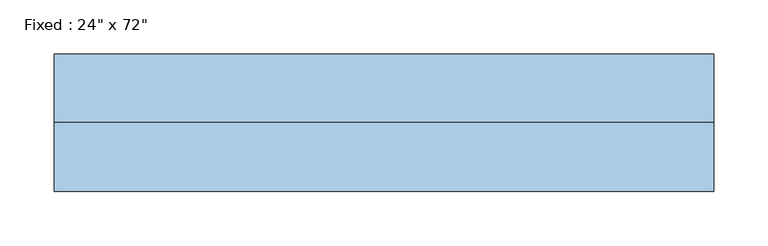
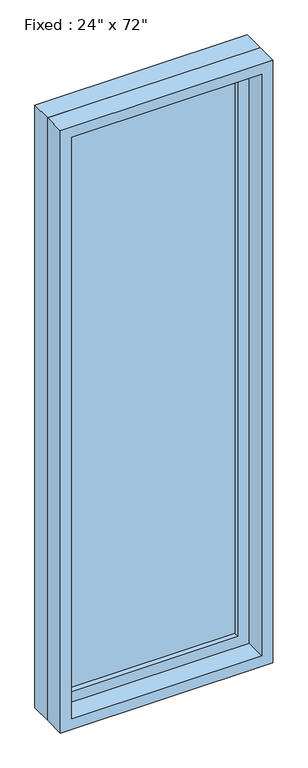
"""IFC4 building model written with IfcOpenShell, lengths in millimetres: window geometry."""

from ifc_helpers import new_model, si_unit, frame, origin, place, context, project, spatial, polyline, outline, extrude, source, transform, mapped, element, save


def window_0bf3737e(model_context):
    return source(origin(), model_context, "Body", "SweptSolid", [
        extrude(outline(polyline([(203.2, 15.875), (-279.4, 15.875), (-279.4, 28.575), (203.2, 28.575), (203.2, 15.875)])), frame((0.0, 0.0, 368.3), z_axis=(0.0, 0.0, 1.0), x_axis=(1.0, 0.0, 0.0)), (0.0, 0.0, 1.0), 1701.8),
        extrude(outline(polyline([(2114.55, -323.85), (323.85, -323.85), (323.85, 247.65), (2114.55, 247.65), (2114.55, -323.85)]), holes=[polyline([(2070.1, -279.4), (2070.1, 203.2), (368.3, 203.2), (368.3, -279.4), (2070.1, -279.4)])]), frame((0.0, 0.0, 0.0), z_axis=(0.0, 1.0, 0.0), x_axis=(0.0, 0.0, 1.0)), (0.0, 0.0, 1.0), 44.45),
        extrude(outline(polyline([(2133.6, -342.9), (304.8, -342.9), (304.8, 266.7), (2133.6, 266.7), (2133.6, -342.9)]), holes=[polyline([(2101.85, -311.15), (2101.85, 234.95), (336.55, 234.95), (336.55, -311.15), (2101.85, -311.15)])]), frame((0.0, -63.5, 0.0), z_axis=(0.0, 1.0, 0.0), x_axis=(0.0, 0.0, 1.0)), (0.0, 0.0, 1.0), 63.5),
        extrude(outline(polyline([(2133.6, 266.7), (2133.6, -342.9), (304.8, -342.9), (304.8, 266.7), (2133.6, 266.7)]), holes=[polyline([(2114.55, 247.65), (323.85, 247.65), (323.85, -323.85), (2114.55, -323.85), (2114.55, 247.65)])]), frame((0.0, 0.0, 0.0), z_axis=(0.0, 1.0, 0.0), x_axis=(0.0, 0.0, 1.0)), (0.0, 0.0, 1.0), 63.5),
    ])


if __name__ == "__main__":
    model = new_model("IFC4")
    model_context = context("Model", 3, world=origin())
    ifc_project = project(units=[si_unit("LENGTHUNIT", "METRE", prefix="MILLI")], contexts=[model_context])
    site = spatial("IfcSite", under=ifc_project)
    building = spatial("IfcBuilding", under=site)
    placement = place(None, origin())
    window_shape = window_0bf3737e(model_context)
    element("IfcWindow", 1, ObjectType="Fixed : 24\" x 72\"", at=placement, inside=building, context=model_context, shape_type="MappedRepresentation", body=[
        mapped(window_shape, transform((0.0, 0.0, 0.0), x_axis=(1.0, 0.0, 0.0), y_axis=(0.0, 1.0, 0.0), z_axis=(0.0, 0.0, 1.0))),
    ])
    save(model, "model.ifc")

# Revit data of these elements
# Type "Fixed : 24\" x 72\""
#   Type Mark = "7"
#   Construction Type Id = "GSP4R"
#   Assembly Code = "B2020100"
#   Analytic Construction = "1/8 in Pilkington single glazing"
#   Visual Light Transmittance = 0.9
#   Solar Heat Gain Coefficient = 0.78
#   Heat Transfer Coefficient (U) = 0.6496 BTU/(h·ft²·°F)
#   Height = 6' - 0"
#   Default Sill Height = 1' - 0"
#   Width = 2' - 0"
#   Window Inset = 0' - 0 3/4"
#   Define Thermal Properties by = 1
#   Define Thermal Properties by = 1
#   Glass Pane Material = Glass
#   Sash Material = Sash
#   Wall Closure = (empty or 0)
# Element 1 (IfcWindow, "Fixed : 24\" x 72\"")
#   Materials on its faces: "Sash", "Glass"
# Materials
#   "Glass": class "Glass", colour RGB 0 128 192, transparency 0.75, Description = "Soda Lime Glass", Cost = 0
#   "Sash": class "Wood", colour RGB 224 178 126, transparency 0, Cost = 0
